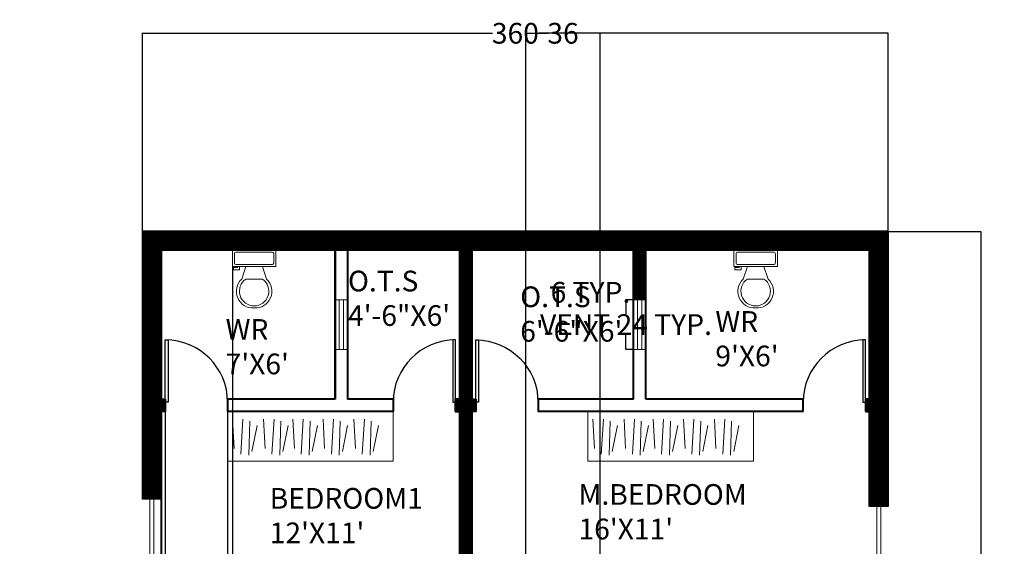
# Model space of a CAD drawing. Units: inches. Extents: x 345 to 1363, y 285 to 1014.
# Tile 4 of 4: x 824 to 1299, y 760 to 1014. Entities that reach past the tile are written whole.
import ezdxf

# ---------------------------------------------------------------- set-up
doc = ezdxf.new("R2010")
doc.units = ezdxf.units.IN
doc.header["$MEASUREMENT"] = 0
for name, color, linetype, lineweight in [('A-ANNO-DIMS', 2, 'Continuous', 18), ('A-AREA-IDEN', 7, 'Continuous', 18), ('A-FLOR-CASE', 8, 'Continuous', 18), ('A-FLOR-FIXT', 9, 'Continuous', 18), ('A-GLAZ', 4, 'Continuous', 18), ('A-WALL', 7, 'Continuous', 40), ('A-WALL-PATT', 252, 'Continuous', 9), ('DOOR', 4, 'Continuous', 25)]:
    doc.layers.add(name, color=color, linetype=linetype, lineweight=lineweight)
doc.styles.get("Standard").update_dxf_attribs({"font": 'arial.ttf'})
doc.dimstyles.get("Standard").update_dxf_attribs({"dimtxt": 10, "dimasz": 0.18, "dimexe": 0.18, "dimexo": 0.0625, "dimgap": 0.09, "dimtad": 0, "dimtih": 1, "dimtoh": 1, "dimdec": 0, "dimzin": 0, "dimdsep": 46, "dimlunit": 3, "dimtxsty": 'Standard', "dimcen": 0.09, "dimadec": 0, "dimazin": 0, "dimtfac": 1, "dimtdec": 0, "dimtofl": 0, "dimtmove": 0, "dimatfit": 3, "dimfxl": 1, "dimtolj": 1, "dimtzin": 0, "dimarcsym": 0})

# ---------------------------------------------------------------- blocks, each defined once
blk = doc.blocks.new('*U4')
for p, q in [((0, 0), (0, -6)), ((40, 0), (40, -6))]:
    blk.add_line(p, q)
blk.add_lwpolyline([(0, 0), (0, 40), (1.75, 40), (1.75, 0)], close=True)
blk.add_arc((0, 0), 40, 0, 90)
blk = doc.blocks.new('*U8')
for p, q in [((0, 0), (0, -6)), ((-40, 0), (-40, -6))]:
    blk.add_line(p, q)
blk.add_lwpolyline([(0, 0), (0, 40), (-1.75, 40), (-1.75, 0)], close=True)
blk.add_arc((0, 0), 40, 90, 180)
blk = doc.blocks.new('*U6')
for p, q in [((9.5, -6), (9.5, -2)), ((-10, -8.5), (-8, -8.5)), ((-10, -9.5), (-10, -8.5)), ((-7, -9.5), (-10, -9.5)), ((-8, -8.5), (-8, -8)), ((-7, -8), (-7, -9.5)), ((-4, -8), (-6, -14)), ((4, -8), (6, -14)), ((4, -14), (-4, -14))]:
    blk.add_line(p, q)
blk.add_lwpolyline([(10.5, -8), (10.5, 0), (-10.5, 0), (-10.5, -8)], close=True)
for points in [[(-9.5, -2), (-9.5, -6)], [(8.5, -1), (-8.5, -1)], [(-8.5, -7), (8.5, -7)]]:
    blk.add_lwpolyline(points)
for centre, radius, start, end in [((-8.625, -1.875), 0.8839, 81.8699, 188.1301), ((8.625, -1.875), 0.8839, 351.8699, 98.1301), ((-8.625, -6.125), 0.8839, 171.869898, 278.1301), ((8.625, -6.125), 0.8839, 261.8699, 8.1301), ((-0.4772, -19.9188), 8.0953, 133.01722, 273.38), ((0.0374, -19.8731), 7.127, 124.50543, 269.7), ((-0.0373, -19.8731), 7.127, 270.3, 55.4946), ((0.4773, -19.9188), 8.0953, 266.62, 46.9828)]:
    blk.add_arc(centre, radius, start, end)
blk = doc.blocks.new('WIN-48IN-EXT')
for p, q in [((9, 48), (0, 48)), ((3.5, 0), (3.5, 48)), ((5.5, 0), (5.5, 48)), ((9, 0), (0, 0))]:
    blk.add_line(p, q)
blk = doc.blocks.new('WIN-24IN-VENT')
for p, q in [((0, 24), (6, 24)), ((2, 24), (2, 0)), ((4, 24), (4, 0)), ((0, 0), (6, 0))]:
    blk.add_line(p, q)
blk = doc.blocks.new('WARDROBE-80X24')
for p, q in [((0, 0), (0, 24)), ((80, 0), (80, 24)), ((2.45, 20.28), (3.21, 6.18)), ((7.49, 20.28), (6.48, 3.41)), ((10.77, 19.28), (10.26, 2.91)), ((17.45, 20.28), (18.2, 6.18)), ((22.49, 20.28), (21.48, 3.41)), ((25.77, 19.28), (25.26, 2.91)), ((31.55, 20.28), (32.31, 6.18)), ((36.59, 20.28), (35.59, 3.41)), ((39.87, 19.28), (39.37, 2.91)), ((46.16, 20.28), (46.91, 6.18)), ((51.2, 20.28), (50.19, 3.41)), ((54.47, 19.28), (53.97, 2.91)), ((61.07, 20.28), (61.83, 6.18)), ((66.11, 20.28), (65.1, 3.41)), ((69.39, 19.28), (68.88, 2.91)), ((14.3, 17.26), (11.77, 4.67)), ((29.29, 17.26), (26.77, 4.67)), ((43.4, 17.26), (40.88, 4.67)), ((58, 17.26), (55.48, 4.67)), ((72.92, 17.26), (70.4, 4.67)), ((80, 0), (0, 0))]:
    blk.add_line(p, q)
blk = doc.blocks.new('*D18')
at = {"layer": 'A-ANNO-DIMS', "color": 0, "lineweight": -2, "transparency": 16777216}
for p, q in [((1120.32, 878.76), (1116.6, 878.76)), ((1116.78, 878.58), (1116.78, 871.88)), ((1116.78, 854.94), (1116.78, 861.65)), ((1120.32, 854.76), (1116.6, 854.76))]:
    blk.add_line(p, q, dxfattribs=at)
at = {"layer": 'A-ANNO-DIMS', "color": 0, "transparency": 16777216}
for points in [[(1116.75, 878.58), (1116.81, 878.58), (1116.78, 878.76)], [(1116.75, 854.94), (1116.81, 854.94), (1116.78, 854.76)]]:
    blk.add_solid(points, dxfattribs=at)
at = {"layer": 'Defpoints', "color": 0, "transparency": 16777216}
for p in [(1120.38, 878.76), (1116.78, 854.76), (1120.38, 854.76)]:
    blk.add_point(p, dxfattribs=at)
at = {"layer": 'A-ANNO-DIMS', "color": 0, "transparency": 16777216, "insert": (1116.78, 866.76), "char_height": 10, "attachment_point": 5}
blk.add_mtext('\\A1;VENT 24 TYP.', dxfattribs=at)
blk = doc.blocks.new('*D19')
at = {"layer": 'A-ANNO-DIMS', "color": 0, "lineweight": -2, "transparency": 16777216}
for p, q in [((1120.38, 882.36), (1120.2, 882.36)), ((1120.38, 878.83), (1120.38, 882.54)), ((1126.2, 882.36), (1120.56, 882.36)), ((1126.38, 878.83), (1126.38, 882.54))]:
    blk.add_line(p, q, dxfattribs=at)
at = {"layer": 'A-ANNO-DIMS', "color": 0, "transparency": 16777216}
for points in [[(1120.56, 882.39), (1120.56, 882.33), (1120.38, 882.36)], [(1126.2, 882.39), (1126.2, 882.33), (1126.38, 882.36)]]:
    blk.add_solid(points, dxfattribs=at)
at = {"layer": 'Defpoints', "color": 0, "transparency": 16777216}
for p in [(1120.38, 882.36), (1120.38, 878.76), (1126.38, 878.76)]:
    blk.add_point(p, dxfattribs=at)
at = {"layer": 'A-ANNO-DIMS', "color": 0, "transparency": 16777216, "insert": (1099.63, 882.36), "char_height": 10, "attachment_point": 5}
blk.add_mtext('\\A1;6 TYP.', dxfattribs=at)
blk = doc.blocks.new('*D32')
at = {"layer": 'A-ANNO-DIMS', "color": 0, "lineweight": -2, "transparency": 16777216}
for p, q in [((883.38, 911.83), (883.38, 1007.64)), ((883.56, 1007.46), (1052.27, 1007.46)), ((1243.2, 1007.46), (1074.5, 1007.46)), ((1243.38, 911.83), (1243.38, 1007.64))]:
    blk.add_line(p, q, dxfattribs=at)
at = {"layer": 'A-ANNO-DIMS', "color": 0, "transparency": 16777216}
for points in [[(883.56, 1007.49), (883.56, 1007.43), (883.38, 1007.46)], [(1243.2, 1007.49), (1243.2, 1007.43), (1243.38, 1007.46)]]:
    blk.add_solid(points, dxfattribs=at)
at = {"layer": 'Defpoints', "color": 0, "transparency": 16777216}
for p in [(1243.38, 1007.46), (883.38, 911.76), (1243.38, 911.76)]:
    blk.add_point(p, dxfattribs=at)
at = {"layer": 'A-ANNO-DIMS', "color": 0, "transparency": 16777216, "insert": (1063.38, 1007.46), "char_height": 10, "attachment_point": 5}
blk.add_mtext('\\A1;360', dxfattribs=at)
blk = doc.blocks.new('*D33')
at = {"layer": 'A-ANNO-DIMS', "color": 0, "lineweight": -2, "transparency": 16777216}
for p, q in [((1243.44, 911.76), (1288.26, 911.76)), ((1288.08, 911.58), (1288.08, 628.96)), ((1288.08, 335.94), (1288.08, 618.57)), ((964.44, 335.76), (1288.26, 335.76))]:
    blk.add_line(p, q, dxfattribs=at)
at = {"layer": 'A-ANNO-DIMS', "color": 0, "transparency": 16777216}
for points in [[(1288.05, 911.58), (1288.11, 911.58), (1288.08, 911.76)], [(1288.05, 335.94), (1288.11, 335.94), (1288.08, 335.76)]]:
    blk.add_solid(points, dxfattribs=at)
at = {"layer": 'Defpoints', "color": 0, "transparency": 16777216}
for p in [(1243.38, 911.76), (1288.08, 911.76), (964.38, 335.76)]:
    blk.add_point(p, dxfattribs=at)
at = {"layer": 'A-ANNO-DIMS', "color": 0, "transparency": 16777216, "insert": (1288.08, 623.76), "char_height": 10, "attachment_point": 5}
blk.add_mtext('\\A1;576', dxfattribs=at)
blk = doc.blocks.new('*D41')
at = {"layer": 'A-ANNO-DIMS', "color": 0, "lineweight": -2, "transparency": 16777216}
for p, q in [((894.38, 824.7), (894.38, 290.88)), ((924.38, 824.7), (924.38, 290.88)), ((894.56, 291.06), (902.15, 291.06)), ((924.2, 291.06), (916.61, 291.06))]:
    blk.add_line(p, q, dxfattribs=at)
at = {"layer": 'A-ANNO-DIMS', "color": 0, "transparency": 16777216}
for points in [[(894.56, 291.09), (894.56, 291.03), (894.38, 291.06)], [(924.2, 291.09), (924.2, 291.03), (924.38, 291.06)]]:
    blk.add_solid(points, dxfattribs=at)
at = {"layer": 'Defpoints', "color": 0, "transparency": 16777216}
for p in [(894.38, 824.76), (924.38, 824.76), (924.38, 291.06)]:
    blk.add_point(p, dxfattribs=at)
at = {"layer": 'A-ANNO-DIMS', "color": 0, "transparency": 16777216, "insert": (909.38, 291.06), "char_height": 10, "attachment_point": 5}
blk.add_mtext('\\A1;30', dxfattribs=at)
blk = doc.blocks.new('*D42')
at = {"layer": 'A-ANNO-DIMS', "color": 0, "lineweight": -2, "transparency": 16777216}
for p, q in [((1068.38, 554.83), (1068.38, 1007.64)), ((1068.56, 1007.46), (1079.14, 1007.46)), ((1104.2, 1007.46), (1093.63, 1007.46)), ((1104.38, 554.83), (1104.38, 1007.64))]:
    blk.add_line(p, q, dxfattribs=at)
at = {"layer": 'A-ANNO-DIMS', "color": 0, "transparency": 16777216}
for points in [[(1068.56, 1007.49), (1068.56, 1007.43), (1068.38, 1007.46)], [(1104.2, 1007.49), (1104.2, 1007.43), (1104.38, 1007.46)]]:
    blk.add_solid(points, dxfattribs=at)
at = {"layer": 'Defpoints', "color": 0, "transparency": 16777216}
for p in [(1104.38, 1007.46), (1068.38, 554.76), (1104.38, 554.76)]:
    blk.add_point(p, dxfattribs=at)
at = {"layer": 'A-ANNO-DIMS', "color": 0, "transparency": 16777216, "insert": (1086.38, 1007.46), "char_height": 10, "attachment_point": 5}
blk.add_mtext('\\A1;36', dxfattribs=at)
blk = doc.blocks.new('*D46')
at = {"layer": 'A-ANNO-DIMS', "color": 0, "lineweight": -2, "transparency": 16777216}
for p, q in [((892.381853, 902.701559), (892.381853, 290.884059)), ((926.755051, 894.701559), (926.755051, 290.884059)), ((892.201853, 291.064059), (892.021853, 291.064059)), ((926.935051, 291.064059), (927.115051, 291.064059))]:
    blk.add_line(p, q, dxfattribs=at)
at = {"layer": 'A-ANNO-DIMS', "color": 0, "transparency": 16777216}
for points in [[(892.201853, 291.094059), (892.201853, 291.034059), (892.381853, 291.064059)], [(926.935051, 291.094059), (926.935051, 291.034059), (926.755051, 291.064059)]]:
    blk.add_solid(points, dxfattribs=at)
at = {"layer": 'Defpoints', "color": 0, "transparency": 16777216}
for p in [(892.381853, 902.764059), (926.755051, 894.764059), (926.755051, 291.064059)]:
    blk.add_point(p, dxfattribs=at)
at = {"layer": 'A-ANNO-DIMS', "color": 0, "transparency": 16777216, "insert": (909.568452, 291.064059), "char_height": 10, "attachment_point": 5}
blk.add_mtext('\\A1;34.37', dxfattribs=at)

msp = doc.modelspace()

# ---------------------------------------------------------------- hatches: boundary and pattern name
at = {"layer": 'A-WALL-PATT'}
h = msp.add_hatch(dxfattribs=at)
h.set_pattern_fill('ANSI31', color=256)
h.paths.add_polyline_path([(760.967, 730.806), (751.967, 730.806), (751.967, 692.764), (671.967, 692.764), (598.143, 692.764), (598.143, 686.764), (697.967, 686.764), (697.967, 586.835), (702.4, 586.835, -0.0130342), (703.967, 586.794), (703.967, 686.764), (751.967, 686.764), (751.967, 626.764), (742.74, 626.764), (742.74, 620.764), (751.967, 620.764), (751.967, 554.764), (703.967, 554.764), (703.967, 556.764), (702.4, 556.764), (697.967, 556.764), (697.967, 554.764), (622.228, 554.764), (622.228, 548.764), (751.967, 548.764), (751.967, 479.508), (760.967, 479.508)])
h.paths.add_polyline_path([(760.967, 431.508), (751.967, 431.508), (751.967, 380.764), (583.967, 380.764), (583.967, 548.764), (585.967, 548.764), (585.967, 549.325), (585.967, 554.764), (583.967, 554.764), (577.967, 554.764), (575.967, 554.764), (575.967, 548.764), (577.967, 548.764), (577.967, 371.764), (760.967, 371.764)])
h.paths.add_polyline_path([(409.967, 548.764), (529.967, 548.764), (529.967, 554.764), (511.967, 554.764), (511.967, 654.693), (507.456, 654.693, -0.0123881), (505.967, 654.73), (505.967, 554.764), (409.967, 554.764), (409.967, 596.764), (400.967, 596.764), (400.967, 371.764), (409.967, 371.764)])
h.paths.add_polyline_path([(409.967, 686.764), (505.967, 686.764), (505.967, 684.764), (507.456, 684.764), (511.967, 684.764), (511.967, 686.764), (515.791, 686.764), (515.791, 692.764), (409.967, 692.764), (409.967, 734.364), (400.967, 734.364), (400.967, 644.764), (409.967, 644.764)])
h.paths.add_polyline_path([(559.967, 824.764), (561.801, 824.764), (561.801, 829.275), (561.801, 830.764), (559.967, 830.764), (559.967, 902.764), (637.967, 902.764), (637.967, 878.764), (643.967, 878.764), (643.967, 902.764), (751.967, 902.764), (751.967, 830.764), (749.967, 830.764), (749.967, 829.275), (749.967, 824.764), (751.967, 824.764), (751.967, 778.806), (760.967, 778.806), (760.967, 911.764), (400.967, 911.764), (400.967, 782.364), (409.967, 782.364), (409.967, 824.764), (411.967, 824.764), (411.967, 829.275), (411.967, 830.764), (409.967, 830.764), (409.967, 902.764), (553.967, 902.764), (553.967, 830.764), (552.038, 830.764), (552.038, 829.275), (552.038, 824.764), (553.967, 824.764), (553.967, 692.764), (552.052, 692.764), (552.052, 692.203), (552.052, 686.764), (553.967, 686.764), (559.967, 686.764), (561.882, 686.764), (561.882, 692.764), (559.967, 692.764)])
h.paths.add_polyline_path([(718.74, 626.764), (703.967, 626.764), (703.967, 620.764), (718.74, 620.764)], flags=17)
h.paths.add_polyline_path([(892.382, 824.764), (894.382, 824.764), (894.382, 829.275), (894.382, 830.764), (892.382, 830.764), (892.382, 902.764), (1036.382, 902.764), (1036.382, 830.764), (1034.453, 830.764), (1034.453, 829.275), (1034.453, 824.764), (1036.382, 824.764), (1036.382, 692.764), (1034.467, 692.764), (1034.467, 692.203), (1034.467, 686.764), (1036.382, 686.764), (1042.382, 686.764), (1044.297, 686.764), (1044.297, 692.764), (1042.382, 692.764), (1042.382, 824.764), (1044.216, 824.764), (1044.216, 829.275), (1044.216, 830.764), (1042.382, 830.764), (1042.382, 902.764), (1120.382, 902.764), (1120.382, 878.764), (1126.382, 878.764), (1126.382, 902.764), (1234.382, 902.764), (1234.382, 830.764), (1232.382, 830.764), (1232.382, 829.275), (1232.382, 824.764), (1234.382, 824.764), (1234.382, 778.806), (1243.382, 778.806), (1243.382, 911.764), (883.382, 911.764), (883.382, 782.364), (892.382, 782.364)])
h.paths.add_polyline_path([(1243.382, 730.806), (1234.382, 730.806), (1234.382, 692.764), (1080.382, 692.764), (1080.382, 686.764), (1180.382, 686.764), (1180.382, 586.764), (1186.382, 586.764), (1186.382, 686.764), (1234.382, 686.764), (1234.382, 626.764), (1225.155, 626.764), (1225.155, 620.764), (1234.382, 620.764), (1234.382, 554.764), (1186.382, 554.764), (1186.382, 556.764), (1180.382, 556.764), (1180.382, 554.764), (1104.382, 554.764), (1104.382, 548.764), (1234.382, 548.764), (1234.382, 479.508), (1243.382, 479.508)])
h.paths.add_polyline_path([(892.382, 686.764), (988.382, 686.764), (988.382, 684.764), (989.871, 684.764), (994.382, 684.764), (994.382, 686.764), (998.206, 686.764), (998.206, 692.203, -0.0038664), (998.21, 692.764), (892.382, 692.764), (892.382, 734.364), (883.382, 734.364), (883.382, 644.764), (892.382, 644.764)])
h.paths.add_polyline_path([(1066.382, 548.764), (1068.382, 548.764), (1068.382, 554.764), (1066.382, 554.764), (1060.382, 554.764), (1058.382, 554.764), (1058.382, 548.764), (1060.382, 548.764), (1060.382, 371.764), (1243.382, 371.764), (1243.382, 431.508), (1234.382, 431.508), (1234.382, 380.764), (1154.382, 380.764), (1066.382, 380.764)])
h.paths.add_polyline_path([(1201.155, 626.764), (1186.382, 626.764), (1186.382, 620.764), (1201.155, 620.764)], flags=17)
h.paths.add_polyline_path([(892.382, 596.764), (883.382, 596.764), (883.382, 371.764), (892.382, 371.764), (892.382, 548.764), (1012.382, 548.764), (1012.382, 554.764), (994.382, 554.764), (994.382, 654.764), (988.382, 654.764), (988.382, 554.764), (892.382, 554.764)])

# ---------------------------------------------------------------- linework, layer by layer
at = {"layer": 'A-WALL'}
for p, q in [((1243.382, 911.764), (883.382, 911.764)), ((883.382, 911.764), (883.382, 782.364)), ((1243.382, 778.806), (1243.382, 911.764)), ((1036.382, 902.764), (892.382, 902.764)), ((892.382, 902.764), (892.382, 830.764)), ((976.382, 902.764), (976.382, 830.764)), ((976.382, 830.764), (976.382, 902.764)), ((982.382, 902.764), (982.382, 830.764)), ((1036.382, 902.764), (1036.382, 830.764)), ((1120.382, 902.764), (1042.382, 902.764)), ((1042.382, 902.764), (1042.382, 830.764)), ((1120.382, 830.764), (1120.382, 902.764)), ((1126.382, 830.764), (1126.382, 902.764)), ((1234.382, 902.764), (1126.382, 902.764)), ((1234.382, 830.764), (1234.382, 902.764)), ((892.382, 830.764), (894.382, 830.764)), ((894.382, 830.764), (894.382, 824.764)), ((976.382, 830.764), (924.382, 830.764)), ((924.382, 830.764), (924.382, 824.764)), ((1004.382, 830.764), (982.382, 830.764)), ((1004.382, 830.764), (1004.382, 824.764)), ((1036.382, 830.764), (1034.382, 830.764)), ((1034.382, 830.764), (1034.382, 824.764)), ((1042.382, 830.764), (1044.382, 830.764)), ((1044.216, 830.764), (1044.216, 824.764)), ((1120.382, 830.764), (1074.382, 830.764)), ((1074.382, 830.764), (1074.382, 824.764)), ((1202.382, 830.764), (1126.382, 830.764)), ((1202.382, 824.764), (1202.382, 830.764)), ((1234.382, 830.764), (1232.382, 830.764)), ((1232.382, 830.764), (1232.382, 824.764)), ((892.382, 824.764), (892.382, 692.764)), ((894.382, 824.764), (892.382, 824.764)), ((1004.382, 824.764), (924.382, 824.764)), ((1034.382, 824.764), (1036.382, 824.764)), ((1036.382, 824.764), (1036.382, 692.764)), ((1042.382, 824.764), (1042.382, 692.764)), ((1044.382, 824.764), (1042.382, 824.764)), ((1202.382, 824.764), (1074.382, 824.764)), ((1232.382, 824.764), (1234.382, 824.764)), ((1234.382, 778.806), (1234.382, 824.764))]:
    msp.add_line(p, q, dxfattribs=at)

# ---------------------------------------------------------------- block references
at = {"layer": 'A-FLOR-CASE'}
for p in [(924.382, 800.764), (1098.382, 800.764)]:
    msp.add_blockref('WARDROBE-80X24', p, dxfattribs=at)
at = {"layer": 'A-FLOR-FIXT'}
for p in [(937.255, 902.764), (1179.401, 902.764)]:
    msp.add_blockref('*U6', p, dxfattribs=at)
at = {"layer": 'A-GLAZ'}
for name, p in [('WIN-24IN-VENT', (976.382, 854.764)), ('WIN-48IN-EXT', (883.382, 734.364)), ('WIN-48IN-EXT', (1234.382, 730.806))]:
    msp.add_blockref(name, p, dxfattribs=at)
at = {"layer": 'A-GLAZ', "rotation": 180}
msp.add_blockref('WIN-24IN-VENT', (1126.382, 878.764), dxfattribs=at)
at = {"layer": 'DOOR', "yscale": 0.7517678943473934, "zscale": 0.7517678943473934}
for name, p, xscale in [('*U4', (894.382, 829.275), 0.7517678943473934), ('*U8', (1034.453, 829.275), 0.7517678943473934), ('*U8', (1044.216, 829.275), -0.7517678943473934), ('*U8', (1232.382, 829.275), 0.7517678943473934)]:
    msp.add_blockref(name, p, dxfattribs=dict(at, xscale=xscale))

# ---------------------------------------------------------------- texts
at = {"layer": 'A-AREA-IDEN', "char_height": 10, "attachment_point": 1}
for s, insert in [('O.T.S\\P4\'-6"X6\'', (982.562, 892.783)), ('O.T.S\\P6\'-6"X6\'', (1065.729, 885.171)), ("WR\\P9'X6'", (1159.935, 873.248)), ("WR\\P7'X6'", (923.498, 869.418)), ("M.BEDROOM\\P16'X11'", (1093.855, 789.691)), ("BEDROOM1\\P12'X11'", (944.775, 787.808))]:
    msp.add_mtext_dynamic_manual_height_columns(s, width=177.75817, gutter_width=1, heights=[0], dxfattribs=dict(at, insert=insert))

# ---------------------------------------------------------------- dimensions: what is measured, and where the dimension line sits
at = {"layer": 'A-ANNO-DIMS'}
for base, p1, p2, override, picture, middle in [((1243.382, 1007.464), (883.382, 911.764), (1243.382, 911.764), {"dimdec": 0, "dimlfac": 1, "dimrnd": 0, "dimzin": 0, "dimdsep": 46, "dimlunit": 2}, '*D32', (1063.382, 1007.464)), ((1104.382, 1007.464), (1068.382, 554.764), (1104.382, 554.764), {"dimdec": 0, "dimlfac": 1, "dimrnd": 0, "dimzin": 0, "dimdsep": 46, "dimlunit": 2}, '*D42', (1086.382, 1007.464)), ((926.755, 291.064), (892.382, 902.764), (926.755, 894.764), {"dimdec": 2, "dimlfac": 1, "dimrnd": 0, "dimzin": 0, "dimdsep": 46, "dimlunit": 2}, '*D46', (909.568, 291.064)), ((924.382, 291.064), (894.382, 824.764), (924.382, 824.764), {"dimdec": 0, "dimlfac": 1, "dimrnd": 0, "dimzin": 0, "dimdsep": 46, "dimlunit": 2}, '*D41', (909.382, 291.064))]:
    dim = msp.add_linear_dim(base=base, p1=p1, p2=p2, dimstyle='Standard', override=override, dxfattribs=at)
    dim.commit()
    dim.dimension.update_dxf_attribs({"geometry": picture, "text_midpoint": middle})
dim = msp.add_linear_dim(base=(1288.082, 911.764), p1=(964.382, 335.764), p2=(1243.382, 911.764), angle=90, dimstyle='Standard', override={"dimdec": 0, "dimlfac": 1, "dimrnd": 0, "dimzin": 0, "dimdsep": 46, "dimlunit": 2}, dxfattribs=at)
dim.commit()
dim.dimension.update_dxf_attribs({"geometry": '*D33', "text_midpoint": (1288.082, 623.764)})
for base, p1, p2, angle, text, picture, middle in [((1120.382, 882.364), (1126.382, 878.764), (1120.382, 878.764), 180, '<> TYP.', '*D19', (1099.631, 882.364)), ((1116.782, 854.764), (1120.382, 878.764), (1120.382, 854.764), 270, 'VENT <> TYP.', '*D18', (1116.782, 866.764))]:
    dim = msp.add_linear_dim(base=base, p1=p1, p2=p2, angle=angle, text=text, dimstyle='Standard', override={"dimdec": 0, "dimlfac": 1, "dimrnd": 0, "dimzin": 0, "dimdsep": 46, "dimlunit": 2}, dxfattribs=at)
    dim.commit()
    dim.dimension.update_dxf_attribs({"geometry": picture, "text_midpoint": middle})

doc.saveas('drawing.dxf')
